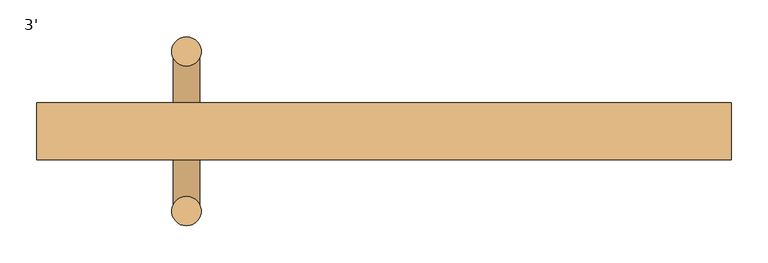
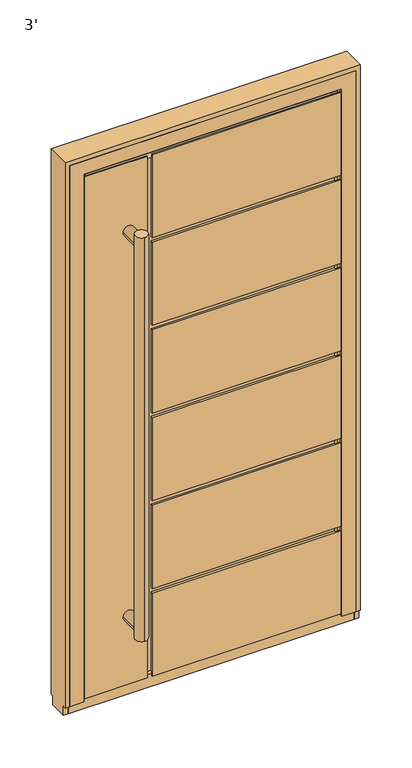
"""IFC4 building model written with IfcOpenShell, lengths in millimetres: door geometry, 3'."""

from ifc_helpers import new_model, si_unit, point, frame, frame_2d, origin, place, context, project, spatial, circle_curve, trimmed, segment, composite_curve, outline, extrude, faceted_brep, source, transform, mapped, element, save


def door_3_3562bf2b(model_context):
    return source(origin(), model_context, "Body", "SolidModel", [
        extrude(outline(composite_curve([segment(trimmed(circle_curve(frame_2d((-268.65, 52.7003001)), 20.0), [point((-268.65, 32.7003001))], [point((-268.65, 72.7003001))], False, "CARTESIAN"), True, "CONTINUOUS"), segment(trimmed(circle_curve(frame_2d((-268.65, 52.7003001)), 20.0), [point((-268.65, 72.7003001))], [point((-268.65, 32.7003001))], False, "CARTESIAN"), True, "CONTINUOUS")], self_intersect=False)), frame((0.0, 0.0, 210.0000003), z_axis=(0.0, 0.0, 1.0), x_axis=(1.0, 0.0, 0.0)), (0.0, 0.0, 1.0), 1363.8),
        extrude(outline(composite_curve([segment(trimmed(circle_curve(frame_2d((-268.65, -164.3003001)), 20.0), [point((-268.65, -184.3003001))], [point((-268.65, -144.3003001))], False, "CARTESIAN"), True, "CONTINUOUS"), segment(trimmed(circle_curve(frame_2d((-268.65, -164.3003001)), 20.0), [point((-268.65, -144.3003001))], [point((-268.65, -184.3003001))], False, "CARTESIAN"), True, "CONTINUOUS")], self_intersect=False)), frame((0.0, 0.0, 210.0000003), z_axis=(0.0, 0.0, 1.0), x_axis=(1.0, 0.0, 0.0)), (0.0, 0.0, 1.0), 1363.8),
        extrude(outline(composite_curve([segment(trimmed(circle_curve(frame_2d((241.9000003, -268.65)), 18.0), [point((241.9000003, -286.65))], [point((241.9000003, -250.65))], False, "CARTESIAN"), True, "CONTINUOUS"), segment(trimmed(circle_curve(frame_2d((241.9000003, -268.65)), 18.0), [point((241.9000003, -250.65))], [point((241.9000003, -286.65))], False, "CARTESIAN"), True, "CONTINUOUS")], self_intersect=False)), frame((0.0, -164.3, 0.0), z_axis=(0.0, 1.0, 0.0), x_axis=(0.0, 0.0, 1.0)), (0.0, 0.0, 1.0), 217.0),
        extrude(outline(composite_curve([segment(trimmed(circle_curve(frame_2d((1541.9000003, -268.65)), 18.0), [point((1541.9000003, -286.65))], [point((1541.9000003, -250.65))], False, "CARTESIAN"), True, "CONTINUOUS"), segment(trimmed(circle_curve(frame_2d((1541.9000003, -268.65)), 18.0), [point((1541.9000003, -250.65))], [point((1541.9000003, -286.65))], False, "CARTESIAN"), True, "CONTINUOUS")], self_intersect=False)), frame((0.0, -164.3, 0.0), z_axis=(0.0, 1.0, 0.0), x_axis=(0.0, 0.0, 1.0)), (0.0, 0.0, 1.0), 217.0),
        faceted_brep([(-193.65, -24.3, 306.466667), (383.65, -24.3, 306.466667), (383.65, -24.3, 291.466667), (-193.65, -24.3, 291.466667), (-193.65, -24.3, 35.0), (-208.65, -24.3, 35.0), (-208.65, -24.3, 1748.8000003), (-193.65, -24.3, 1748.8000003), (-193.65, -24.3, 1492.3333337), (383.65, -24.3, 1492.3333337), (383.65, -24.3, 1477.3333337), (-193.65, -24.3, 1477.3333337), (-193.65, -24.3, 1195.866667), (383.65, -24.3, 1195.866667), (383.65, -24.3, 1180.866667), (-193.65, -24.3, 1180.866667), (-193.65, -24.3, 899.4000004), (383.65, -24.3, 899.4000004), (383.65, -24.3, 884.4000004), (-193.65, -24.3, 884.4000004), (-193.65, -24.3, 602.9333337), (383.65, -24.3, 602.9333337), (383.65, -24.3, 587.9333337), (-193.65, -24.3, 587.9333337), (-193.65, -17.3, 587.9333337), (-193.65, -17.3, 306.466667), (383.65, -17.3, 587.9333337), (383.65, -26.3002302, 1748.8000003), (383.65, -26.3002302, 35.0), (383.65, -19.2979528, 35.0), (383.65, -19.2979528, 24.0), (383.65, -17.3, 24.0), (383.65, -17.3, 291.466667), (383.65, -17.3, 306.466667), (383.65, -17.3, 602.9333337), (383.65, -17.3, 884.4000004), (383.65, -17.3, 899.4000004), (383.65, -17.3, 1180.866667), (383.65, -17.3, 1195.866667), (383.65, -17.3, 1477.3333337), (383.65, -17.3, 1492.3333337), (383.65, -17.3, 1748.8000003), (-193.65, -17.3, 602.9333337), (-193.65, -17.3, 884.4000004), (-193.65, -17.3, 899.4000004), (-193.65, -17.3, 1180.866667), (-208.65, -19.2979528, 35.0), (-208.65, -19.2979528, 24.0), (-208.65, -17.3, 24.0), (-208.65, -17.3, 1748.8000003), (-383.65, -26.3002302, 35.0), (-383.65, -19.2979528, 35.0), (-193.65, -19.2979528, 35.0), (-193.65, -17.3, 291.466667), (-193.65, -17.3, 24.0), (-193.65, -19.2979528, 24.0), (-383.65, -19.2979528, 24.0), (-383.65, -17.3, 24.0), (-383.65, -17.3, 1748.8000003), (-193.65, -17.3, 1195.866667), (-193.65, -17.3, 1477.3333337), (-193.65, -17.3, 1492.3333337), (-193.65, -17.3, 1748.8000003), (408.65, -94.3, 10.0000003), (-193.65, -94.3, 10.0000003), (-193.65, -91.3, 10.0000003), (408.65, -91.3, 10.0000003), (-408.65, -91.3, 10.0000003), (-208.65, -91.3, 10.0000003), (-208.65, -94.3, 10.0000003), (-408.65, -94.3, 10.0000003), (408.65, -94.3, 306.466667), (408.65, -91.3, 306.466667), (408.65, -91.3, 587.9333337), (408.65, -94.3, 587.9333337), (408.65, -94.3, 899.4000004), (408.65, -91.3, 899.4000004), (408.65, -91.3, 1180.866667), (408.65, -94.3, 1180.866667), (408.65, -94.3, 602.9333337), (408.65, -91.3, 602.9333337), (408.65, -91.3, 884.4000004), (408.65, -94.3, 884.4000004), (408.65, -94.3, 1195.866667), (408.65, -91.3, 1195.866667), (408.65, -91.3, 1477.3333337), (408.65, -94.3, 1477.3333337), (408.65, -94.3, 1773.8000003), (408.65, -94.3, 1492.3333337), (408.65, -91.3, 1492.3333337), (408.65, -91.3, 1773.8000003), (408.65, -91.3, 291.466667), (408.65, -94.3, 291.466667), (-193.65, -91.3, 25.5), (393.15, -91.3, 25.5), (393.15, -91.3, 291.466667), (393.15, -91.3, 306.466667), (393.15, -91.3, 587.9333337), (393.15, -91.3, 899.4000004), (393.15, -91.3, 1180.866667), (393.15, -91.3, 602.9333337), (393.15, -91.3, 884.4000004), (-393.15, -91.3, 25.5), (-208.65, -91.3, 25.5), (-408.65, -91.3, 1773.8000003), (-208.65, -91.3, 1773.8000003), (-208.65, -91.3, 1758.3000003), (-393.15, -91.3, 1758.3000003), (393.15, -91.3, 1195.866667), (393.15, -91.3, 1477.3333337), (393.15, -91.3, 1492.3333337), (393.15, -91.3, 1758.3000003), (-193.65, -91.3, 1758.3000003), (-193.65, -91.3, 1773.8000003), (-193.65, -87.3, 291.466667), (-193.65, -87.3, 25.5), (-193.65, -94.3, 291.466667), (-208.65, -94.3, 1773.8000003), (-408.65, -94.3, 1773.8000003), (-193.65, -94.3, 587.9333337), (-193.65, -94.3, 306.466667), (-193.65, -94.3, 1180.866667), (-193.65, -94.3, 899.4000004), (-193.65, -94.3, 884.4000004), (-193.65, -94.3, 602.9333337), (-193.65, -94.3, 1477.3333337), (-193.65, -94.3, 1195.866667), (-193.65, -94.3, 1773.8000003), (-193.65, -94.3, 1492.3333337), (-208.65, -87.3, 1758.3000003), (-208.65, -87.3, 25.5), (-383.65, -26.3002302, 1748.8000003), (393.15, -26.3002302, 1758.3000003), (393.15, -26.3002302, 25.5), (-393.15, -26.3002302, 25.5), (-393.15, -26.3002302, 1758.3000003), (393.15, -87.3, 1492.3333337), (393.15, -87.3, 1477.3333337), (393.15, -87.3, 1195.866667), (393.15, -87.3, 1180.866667), (393.15, -87.3, 899.4000004), (393.15, -87.3, 884.4000004), (393.15, -87.3, 602.9333337), (393.15, -87.3, 587.9333337), (393.15, -87.3, 306.466667), (393.15, -87.3, 291.466667), (-193.65, -87.3, 1477.3333337), (-193.65, -87.3, 1492.3333337), (-193.65, -87.3, 1758.3000003), (-193.65, -87.3, 306.466667), (-193.65, -87.3, 587.9333337), (-193.65, -87.3, 602.9333337), (-193.65, -87.3, 884.4000004), (-193.65, -87.3, 899.4000004), (-193.65, -87.3, 1180.866667), (-193.65, -87.3, 1195.866667)], [[[0, 1, 2, 3, 4, 5, 6, 7, 8, 9, 10, 11, 12, 13, 14, 15, 16, 17, 18, 19, 20, 21, 22, 23]], [[23, 24, 25, 0]], [[23, 22, 26, 24]], [[27, 28, 29, 30, 31, 32, 2, 1, 33, 26, 22, 21, 34, 35, 18, 17, 36, 37, 14, 13, 38, 39, 10, 9, 40, 41]], [[42, 34, 21, 20]], [[19, 43, 42, 20]], [[19, 18, 35, 43]], [[44, 36, 17, 16]], [[15, 45, 44, 16]], [[5, 46, 47, 48, 49, 6]], [[28, 50, 51, 46, 5, 4, 52, 29]], [[53, 54, 55, 52, 4, 3]], [[3, 2, 32, 53]], [[25, 33, 1, 0]], [[29, 52, 55, 30]], [[56, 47, 46, 51]], [[30, 55, 54, 31]], [[57, 48, 47, 56]], [[36, 44, 45, 37]], [[34, 42, 43, 35]], [[33, 25, 24, 26]], [[54, 53, 32, 31]], [[58, 49, 48, 57]], [[38, 59, 60, 39]], [[41, 40, 61, 62]], [[63, 64, 65, 66]], [[67, 68, 69, 70]], [[71, 72, 73, 74]], [[75, 76, 77, 78]], [[79, 80, 81, 82]], [[83, 84, 85, 86]], [[87, 88, 89, 90]], [[66, 91, 92, 63]], [[65, 93, 94, 95, 91, 66]], [[72, 96, 97, 73]], [[76, 98, 99, 77]], [[80, 100, 101, 81]], [[102, 103, 68, 67, 104, 105, 106, 107]], [[84, 108, 109, 85]], [[90, 89, 110, 111, 112, 113]], [[114, 115, 93, 65, 64, 116]], [[70, 69, 117, 118]], [[63, 92, 116, 64]], [[74, 119, 120, 71]], [[78, 121, 122, 75]], [[82, 123, 124, 79]], [[86, 125, 126, 83]], [[87, 127, 128, 88]], [[70, 118, 104, 67]], [[129, 106, 105, 117, 69, 68, 103, 130]], [[58, 57, 56, 51, 50, 131]], [[132, 133, 134, 135], [131, 50, 28, 27]], [[111, 110, 136, 137, 109, 108, 138, 139, 99, 98, 140, 141, 101, 100, 142, 143, 97, 96, 144, 145, 95, 94, 133, 132]], [[94, 93, 115, 130, 103, 102, 134, 133]], [[135, 134, 102, 107]], [[146, 137, 136, 147, 148, 129, 130, 115, 114, 145, 144, 149, 150, 143, 142, 151, 152, 141, 140, 153, 154, 139, 138, 155]], [[153, 122, 121, 154]], [[153, 140, 98, 76, 75, 122]], [[123, 82, 81, 101, 141, 152]], [[151, 124, 123, 152]], [[151, 142, 100, 80, 79, 124]], [[119, 74, 73, 97, 143, 150]], [[149, 120, 119, 150]], [[149, 144, 96, 72, 71, 120]], [[116, 92, 91, 95, 145, 114]], [[15, 14, 37, 45]], [[59, 38, 13, 12]], [[11, 60, 59, 12]], [[11, 10, 39, 60]], [[61, 40, 9, 8]], [[8, 7, 62, 61]], [[125, 86, 85, 109, 137, 146]], [[128, 127, 113, 112, 148, 147]], [[121, 78, 77, 99, 139, 154]], [[155, 138, 108, 84, 83, 126]], [[155, 126, 125, 146]], [[147, 136, 110, 89, 88, 128]], [[90, 113, 127, 87]], [[118, 117, 105, 104]], [[132, 135, 107, 106, 129, 148, 112, 111]], [[27, 41, 62, 7, 6, 49, 58, 131]]]),
        faceted_brep([(-457.2, -94.3, 0.0), (-457.2, -85.2997571, 0.0), (-412.7, -85.2997571, 0.0), (-412.7, -94.3, 0.0), (-403.2, -21.8000042, 0.0), (-403.2, -26.3, 0.0), (-457.2, -26.3, 0.0), (-457.2, -17.3, 0.0), (-387.7, -17.3, 0.0), (-387.7, -21.8000042, 0.0), (457.2, -17.3, 0.0), (457.2, -26.3, 0.0), (403.2, -26.3, 0.0), (403.2, -21.8000042, 0.0), (387.7, -21.8000042, 0.0), (387.7, -17.3, 0.0), (412.7, -85.2997571, 0.0), (457.2, -85.2997571, 0.0), (457.2, -94.3, 0.0), (412.7, -94.3, 0.0), (-457.2, -26.3, -30.0), (-457.2, -85.2997571, -30.0), (-457.2, -94.3, 1828.8), (-457.2, -17.3, 1828.8), (-412.7, -94.3, 1784.3), (412.7, -94.3, 1784.3), (457.2, -94.3, 1828.8), (457.2, -17.3, 1828.8), (457.2, -85.2997571, -30.0), (457.2, -26.3, -30.0), (387.7, -17.3, 1759.3), (-387.7, -17.3, 1759.3), (-403.2, -85.3, 1774.8), (-403.2, -85.3, 14.5), (-403.2, -26.3, 14.5), (-403.2, -21.8000042, 1774.8), (403.2, -21.8000042, 1774.8), (403.2, -85.3, 1774.8), (403.2, -26.3, 14.5), (403.2, -85.3, 14.5), (-412.7, -85.3, 1784.3), (412.7, -85.3, 1784.3), (-387.7, -21.8000042, 1759.3), (387.7, -21.8000042, 1759.3)], [[[0, 1, 2, 3]], [[4, 5, 6, 7, 8, 9]], [[10, 11, 12, 13, 14, 15]], [[16, 17, 18, 19]], [[7, 6, 20, 21, 1, 0, 22, 23]], [[3, 24, 25, 19, 18, 26, 22, 0]], [[22, 26, 27, 23]], [[18, 17, 28, 29, 11, 10, 27, 26]], [[7, 23, 27, 10, 15, 30, 31, 8]], [[32, 33, 34, 5, 4, 35]], [[35, 36, 37, 32]], [[36, 13, 12, 38, 39, 37]], [[40, 24, 3, 2]], [[16, 41, 40, 2, 1, 21, 28, 17], [37, 39, 33, 32]], [[9, 42, 43, 14, 13, 36, 35, 4]], [[8, 31, 42, 9]], [[24, 40, 41, 25]], [[30, 43, 42, 31]], [[19, 25, 41, 16]], [[14, 43, 30, 15]], [[20, 6, 5, 34, 38, 12, 11, 29]], [[39, 38, 34, 33]], [[20, 29, 28, 21]]]),
        faceted_brep([(-457.2, -85.3, -30.0), (-472.2, -85.3, -30.0), (-472.2, -26.3, -30.0), (-457.2, -26.3, -30.0), (-457.2, -94.3, 1828.8), (-457.2, -94.3, 0.0), (-457.2, -85.3, 0.0), (-457.2, -26.3, 0.0), (-457.2, -17.3, 0.0), (-457.2, -17.3, 1828.8), (-472.2, -26.3, 0.0), (472.2, -26.3, 0.0), (472.2, -26.3, -30.0), (457.2, -26.3, -30.0), (457.2, -26.3, 0.0), (-472.2, -17.3, 1843.8), (-472.2, -17.3, 0.0), (-472.2, -85.3, 0.0), (-472.2, -94.3, 0.0), (-472.2, -94.3, 1843.8), (457.2, -85.3, 0.0), (457.2, -85.3, -30.0), (472.2, -85.3, -30.0), (472.2, -85.3, 0.0), (457.2, -17.3, 1828.8), (457.2, -17.3, 0.0), (457.2, -94.3, 0.0), (457.2, -94.3, 1828.8), (472.2, -94.3, 0.0), (472.2, -94.3, 1843.8), (472.2, -17.3, 0.0), (472.2, -17.3, 1843.8)], [[[0, 1, 2, 3]], [[4, 5, 6, 0, 3, 7, 8, 9]], [[7, 3, 2, 10]], [[11, 12, 13, 14]], [[15, 16, 10, 2, 1, 17, 18, 19]], [[17, 1, 0, 6]], [[20, 21, 22, 23]], [[24, 25, 14, 13, 21, 20, 26, 27]], [[27, 26, 28, 29, 19, 18, 5, 4]], [[6, 5, 18, 17]], [[23, 28, 26, 20]], [[22, 21, 13, 12]], [[10, 16, 8, 7]], [[14, 25, 30, 11]], [[9, 8, 16, 15, 31, 30, 25, 24]], [[29, 28, 23, 22, 12, 11, 30, 31]], [[9, 24, 27, 4]], [[19, 29, 31, 15]]]),
    ])


if __name__ == "__main__":
    model = new_model("IFC4")
    model_context = context("Model", 3, world=origin())
    ifc_project = project(units=[si_unit("LENGTHUNIT", "METRE", prefix="MILLI")], contexts=[model_context])
    site = spatial("IfcSite", under=ifc_project)
    building = spatial("IfcBuilding", under=site)
    placement = place(None, origin())
    door_3_shape = door_3_3562bf2b(model_context)
    element("IfcDoor", 1, ObjectType="3'", at=placement, inside=building, context=model_context, shape_type="MappedRepresentation", body=[
        mapped(door_3_shape, transform((0.0, 0.0, 0.0), x_axis=(1.0, 0.0, 0.0), y_axis=(0.0, 1.0, 0.0), z_axis=(0.0, 0.0, 1.0))),
    ])
    save(model, "model.ifc")

# Revit data of these elements
# Type "3'"
#   Type Mark = "9"
#   Water resistance = "up to Class E900, EN 12208:2001"
#   Uniclass2015Version = "v1.21"
#   Uniclass2015Reference = "Ss_25_30_20_30"
#   Uniclass2015Description = "Frame and door leaf system"
#   URL = "www.aluprof.com"
#   Type IFC Predefined Type = "USERDEFINED"
#   Right-hand / Left-hand door [instance default] = ""
#   Resistance to wind load = "up to Class C5/B5, EN 12210:2001"
#   Insert type = "ST"
#   Hardware [instance default] = ""
#   Product page = "https://aluprof.com/en/architects/offer/window-and-door-systems/panel-doors#visualisation"
#   Operation = "SinglePanelOutwardOpening"
#   Opening type = "Outward"
#   NBSReference = "25-50-20/125"
#   NBSDescription = "Frame and door leaf system"
#   Important = "The actual acceptable construction dimensions are dependent on the selection of profiles and hardware, glazing type, construction weight and the construction’s operating conditions. These should be determined by a suitably qualified person, and using ALUPROF’s calculation software"
#   IfcExportType = "USERDEFINED"
#   IfcExportAs = "IfcDoorType"
#   Handle type [instance default] = ""
#   Manufacturer = "ALUPROF SA"
#   Export Type to IFC As = "IfcDoorType"
#   Door sill type [instance default] = ""
#   Description = "External single-leaf panel door outward opening"
#   Model = "MB-86 ST Panel Door AD07"
#   Content of the recyclate in the material = "69.2%"
#   COBie.Type.WarrantyDurationParts = ""
#   COBie.Type.Name = ""
#   COBie.Type.Manufacturer = "ALUPROF SA"
#   COBie.Space.Name = ""
#   COBie.Floor.Name = ""
#   COBie.Facility.Name = ""
#   COBie.CreatedOn = ""
#   COBie.Component.WarrantyStartDate = ""
#   COBie.Component.Name = "MB-86 ST Panel Door AD07"
#   Burglar resistance = "RC2"
#   Air permeability = "up to Class 4, EN 12207:2001"
#   Width of the active leaf = 2' - 8.17717"
#   Placement in wall = 0' - 0.7874"
#   Thickness = 0' - 3.0315"
#   Height of the opening sash = 5' - 9.44094"
#   Handle Offset = 3' - 5.33858"
#   Rough Height = 6' - 2.40945"
#   Rough Width = 3' - 1.1811"
#   Height = 6' - 0"
#   Width = 3' - 0"
#   Construction depth = 0' - 3.0315"
#   Clear opening width = 2' - 3.94882"
#   Clear opening height = 5' - 8.47638"
#   Height of the array = 0' - 11.08136"
#   Schedule No. [instance default] = 1
#   Handrail [instance default] = yes
#   IsExternal = yes
#   Handle [instance default] = no
#   Door closer [instance default] = no
#   Function = 1
#   COBie.Type = yes
#   COBie = yes
#   Access control [instance default] = no
#   Panel = element 380416
#   Wall Closure = (empty or 0)
